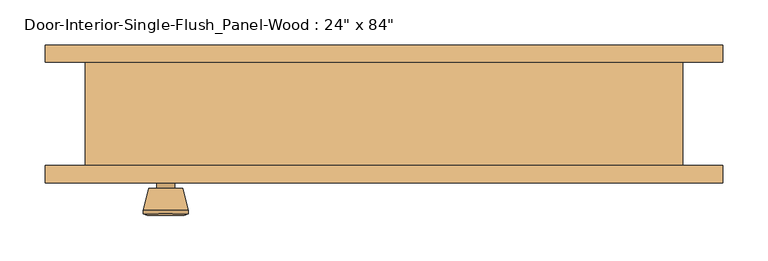
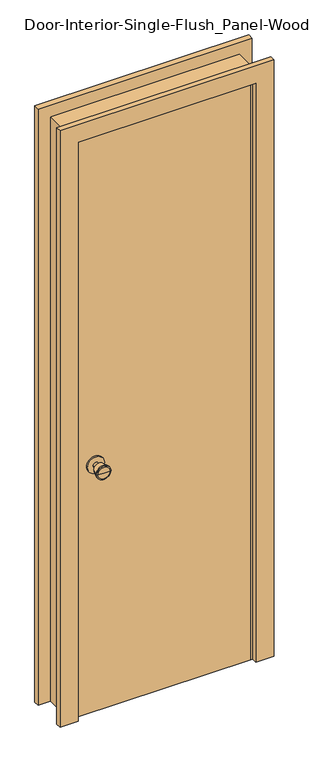
"""IFC4 building model written with IfcOpenShell, lengths in millimetres: door geometry."""

from ifc_helpers import new_model, si_unit, point, frame, frame_2d, origin, origin_with_axes, place, context, project, spatial, polyline, circle_curve, trimmed, segment, composite_curve, outline, extrude, faceted_brep, source, transform, mapped, element, save
from ifc_brep_helpers import plane_surface, cylinder_surface, revolved_surface, advanced_brep


def door_03233f92(model_context):
    return source(origin(), model_context, "Body", "SolidModel", [
        advanced_brep(
        [(-241.3, -13.05, 914.4), (-251.3, -13.05, 914.4), (-231.3, -13.05, 914.4), (-220.8241324, 35.95, 914.4), (-261.7758676, 35.95, 914.4), (-241.3, 35.95, 914.4), (-216.3, 34.1221319, 914.4), (-266.3, 34.1221319, 914.4), (-216.3, 30.6584537, 914.4), (-266.3, 30.6584537, 914.4), (-222.663764, 5.95, 914.4), (-259.936236, 5.95, 914.4), (-231.3, 5.95, 914.4), (-251.3, 5.95, 914.4)],
        [
            (0, 1),
            (1, 2, circle_curve(frame((-241.3, -13.05, 914.4), z_axis=(0.0, -1.0, 0.0), x_axis=(-1.0, 0.0, 0.0)), 10.0)),
            (2, 0),
            (2, 1, circle_curve(frame((-241.3, -13.05, 914.4), z_axis=(0.0, -1.0, 0.0), x_axis=(-1.0, 0.0, 0.0)), 10.0)),
            (3, 4, circle_curve(frame((-241.3, 35.95, 914.4), z_axis=(0.0, 1.0, 0.0), x_axis=(-1.0, 0.0, 0.0)), 20.4758676)),
            (4, 5),
            (5, 3),
            (4, 3, circle_curve(frame((-241.3, 35.95, 914.4), z_axis=(0.0, 1.0, 0.0), x_axis=(-1.0, 0.0, 0.0)), 20.4758676)),
            (6, 7, circle_curve(frame((-241.3, 34.1221319, 914.4), z_axis=(0.0, 1.0, 0.0), x_axis=(-1.0, 0.0, 0.0)), 25.0)),
            (7, 4),
            (3, 6),
            (7, 6, circle_curve(frame((-241.3, 34.1221319, 914.4), z_axis=(0.0, 1.0, 0.0), x_axis=(-1.0, 0.0, 0.0)), 25.0)),
            (8, 9, circle_curve(frame((-241.3, 30.6584537, 914.4), z_axis=(0.0, 1.0, 0.0), x_axis=(-1.0, 0.0, 0.0)), 25.0)),
            (9, 7),
            (6, 8),
            (9, 8, circle_curve(frame((-241.3, 30.6584537, 914.4), z_axis=(0.0, 1.0, 0.0), x_axis=(-1.0, 0.0, 0.0)), 25.0)),
            (10, 11, circle_curve(frame((-241.3, 5.95, 914.4), z_axis=(0.0, 1.0, 0.0), x_axis=(-1.0, 0.0, 0.0)), 18.636236)),
            (11, 9),
            (8, 10),
            (11, 10, circle_curve(frame((-241.3, 5.95, 914.4), z_axis=(0.0, 1.0, 0.0), x_axis=(-1.0, 0.0, 0.0)), 18.636236)),
            (12, 13, circle_curve(frame((-241.3, 5.95, 914.4), z_axis=(0.0, 1.0, 0.0), x_axis=(-1.0, 0.0, 0.0)), 10.0)),
            (13, 11),
            (10, 12),
            (13, 12, circle_curve(frame((-241.3, 5.95, 914.4), z_axis=(0.0, 1.0, 0.0), x_axis=(-1.0, 0.0, 0.0)), 10.0)),
            (1, 13),
            (12, 2),
        ],
        [
            plane_surface(frame((-241.3, -13.05, 914.4), z_axis=(0.0, -1.0, 0.0), x_axis=(-1.0, 0.0, 0.0))),
            plane_surface(frame((-241.3, 35.95, 914.4), z_axis=(0.0, 1.0, 0.0), x_axis=(-1.0, 0.0, 0.0))),
            revolved_surface(polyline([(-261.7758676, 35.95, 914.4), (-266.3, 34.1221319, 914.4)]), (-241.3, -13.05, 914.4), (0.0, -1.0, 0.0)),
            cylinder_surface(frame((-241.3, -13.05, 914.4), z_axis=(0.0, -1.0, 0.0), x_axis=(-1.0, 0.0, 0.0)), 25.0),
            revolved_surface(polyline([(-266.3, 30.6584537, 914.4), (-259.936236, 5.95, 914.4)]), (-241.3, -13.05, 914.4), (0.0, -1.0, 0.0)),
            plane_surface(frame((-241.3, 5.95, 914.4), z_axis=(0.0, -1.0, 0.0), x_axis=(-1.0, 0.0, 0.0))),
            cylinder_surface(frame((-241.3, -13.05, 914.4), z_axis=(0.0, -1.0, 0.0), x_axis=(-1.0, 0.0, 0.0)), 10.0),
        ],
        [
            (0, [[1, 2, 3]]),
            (0, [[-3, 4, -1]]),
            (1, [[5, 6, 7]]),
            (1, [[8, -7, -6]]),
            (2, [[9, 10, -5, 11]]),
            (2, [[12, -11, -8, -10]]),
            (3, [[13, 14, -9, 15]]),
            (3, [[16, -15, -12, -14]]),
            (4, [[17, 18, -13, 19]]),
            (4, [[20, -19, -16, -18]]),
            (5, [[21, 22, -17, 23]]),
            (5, [[24, -23, -20, -22]]),
            (6, [[-2, 25, -21, 26]]),
            (6, [[-4, -26, -24, -25]]),
        ],
    ),
        extrude(outline(composite_curve([segment(trimmed(circle_curve(frame_2d((914.4, -241.3)), 30.0), [point((914.4, -271.3))], [point((914.4, -211.3))], False, "CARTESIAN"), True, "CONTINUOUS"), segment(trimmed(circle_curve(frame_2d((914.4, -241.3)), 30.0), [point((914.4, -211.3))], [point((914.4, -271.3))], False, "CARTESIAN"), True, "CONTINUOUS")], self_intersect=False)), frame((0.0, -19.05, 0.0), z_axis=(0.0, 1.0, 0.0), x_axis=(0.0, 0.0, 1.0)), (0.0, 0.0, 1.0), 6.0),
        advanced_brep(
        [(-241.3, -59.975, 914.4), (-231.3, -59.975, 914.4), (-251.3, -59.975, 914.4), (-220.8241324, -108.975, 914.4), (-241.3, -108.975, 914.4), (-261.7758676, -108.975, 914.4), (-216.3, -107.1471319, 914.4), (-266.3, -107.1471319, 914.4), (-216.3, -103.6834537, 914.4), (-266.3, -103.6834537, 914.4), (-222.663764, -78.975, 914.4), (-259.936236, -78.975, 914.4), (-231.3, -78.975, 914.4), (-251.3, -78.975, 914.4)],
        [
            (0, 1),
            (1, 2, circle_curve(frame((-241.3, -59.975, 914.4), z_axis=(0.0, 1.0, 0.0), x_axis=(-1.0, 0.0, 0.0)), 10.0)),
            (2, 0),
            (2, 1, circle_curve(frame((-241.3, -59.975, 914.4), z_axis=(0.0, 1.0, 0.0), x_axis=(-1.0, 0.0, 0.0)), 10.0)),
            (3, 4),
            (4, 5),
            (5, 3, circle_curve(frame((-241.3, -108.975, 914.4), z_axis=(0.0, -1.0, 0.0), x_axis=(-1.0, 0.0, 0.0)), 20.4758676)),
            (3, 5, circle_curve(frame((-241.3, -108.975, 914.4), z_axis=(0.0, -1.0, 0.0), x_axis=(-1.0, 0.0, 0.0)), 20.4758676)),
            (6, 3),
            (5, 7),
            (7, 6, circle_curve(frame((-241.3, -107.1471319, 914.4), z_axis=(0.0, -1.0, 0.0), x_axis=(-1.0, 0.0, 0.0)), 25.0)),
            (6, 7, circle_curve(frame((-241.3, -107.1471319, 914.4), z_axis=(0.0, -1.0, 0.0), x_axis=(-1.0, 0.0, 0.0)), 25.0)),
            (8, 6),
            (7, 9),
            (9, 8, circle_curve(frame((-241.3, -103.6834537, 914.4), z_axis=(0.0, -1.0, 0.0), x_axis=(-1.0, 0.0, 0.0)), 25.0)),
            (8, 9, circle_curve(frame((-241.3, -103.6834537, 914.4), z_axis=(0.0, -1.0, 0.0), x_axis=(-1.0, 0.0, 0.0)), 25.0)),
            (10, 8),
            (9, 11),
            (11, 10, circle_curve(frame((-241.3, -78.975, 914.4), z_axis=(0.0, -1.0, 0.0), x_axis=(-1.0, 0.0, 0.0)), 18.636236)),
            (10, 11, circle_curve(frame((-241.3, -78.975, 914.4), z_axis=(0.0, -1.0, 0.0), x_axis=(-1.0, 0.0, 0.0)), 18.636236)),
            (12, 10),
            (11, 13),
            (13, 12, circle_curve(frame((-241.3, -78.975, 914.4), z_axis=(0.0, -1.0, 0.0), x_axis=(-1.0, 0.0, 0.0)), 10.0)),
            (12, 13, circle_curve(frame((-241.3, -78.975, 914.4), z_axis=(0.0, -1.0, 0.0), x_axis=(-1.0, 0.0, 0.0)), 10.0)),
            (1, 12),
            (13, 2),
        ],
        [
            plane_surface(frame((-241.3, -59.975, 914.4), z_axis=(0.0, 1.0, 0.0), x_axis=(-1.0, 0.0, 0.0))),
            plane_surface(frame((-241.3, -108.975, 914.4), z_axis=(0.0, -1.0, 0.0), x_axis=(-1.0, 0.0, 0.0))),
            revolved_surface(polyline([(-261.7758676, -108.975, 914.4), (-266.3, -107.1471319, 914.4)]), (-241.3, -59.975, 914.4), (0.0, 1.0, 0.0)),
            cylinder_surface(frame((-241.3, -59.975, 914.4), z_axis=(0.0, 1.0, 0.0), x_axis=(-1.0, 0.0, 0.0)), 25.0),
            revolved_surface(polyline([(-266.3, -103.6834537, 914.4), (-259.936236, -78.975, 914.4)]), (-241.3, -59.975, 914.4), (0.0, 1.0, 0.0)),
            plane_surface(frame((-241.3, -78.975, 914.4), z_axis=(0.0, 1.0, 0.0), x_axis=(-1.0, 0.0, 0.0))),
            cylinder_surface(frame((-241.3, -59.975, 914.4), z_axis=(0.0, 1.0, 0.0), x_axis=(-1.0, 0.0, 0.0)), 10.0),
        ],
        [
            (0, [[1, 2, 3]]),
            (0, [[-3, 4, -1]]),
            (1, [[5, 6, 7]]),
            (1, [[-6, -5, 8]]),
            (2, [[9, -7, 10, 11]]),
            (2, [[-10, -8, -9, 12]]),
            (3, [[13, -11, 14, 15]]),
            (3, [[-14, -12, -13, 16]]),
            (4, [[17, -15, 18, 19]]),
            (4, [[-18, -16, -17, 20]]),
            (5, [[21, -19, 22, 23]]),
            (5, [[-22, -20, -21, 24]]),
            (6, [[25, -23, 26, -2]]),
            (6, [[-26, -24, -25, -4]]),
        ],
    ),
        extrude(outline(composite_curve([segment(trimmed(circle_curve(frame_2d((914.4, -241.3)), 30.0), [point((914.4, -271.3))], [point((914.4, -211.3))], False, "CARTESIAN"), True, "CONTINUOUS"), segment(trimmed(circle_curve(frame_2d((914.4, -241.3)), 30.0), [point((914.4, -211.3))], [point((914.4, -271.3))], False, "CARTESIAN"), True, "CONTINUOUS")], self_intersect=False)), frame((0.0, -59.975, 0.0), z_axis=(0.0, 1.0, 0.0), x_axis=(0.0, 0.0, 1.0)), (0.0, 0.0, 1.0), 6.0),
        faceted_brep([(330.2, -53.975, 0.0), (304.8, -53.975, 0.0), (304.8, -19.05, 0.0), (292.1, -19.05, 0.0), (292.1, 15.875, 0.0), (304.8, 15.875, 0.0), (304.8, 60.325, 0.0), (330.2, 60.325, 0.0), (330.2, 60.325, 2159.0), (330.2, -53.975, 2159.0), (304.8, 60.325, 2133.6), (-304.8, 60.325, 2133.6), (-304.8, 60.325, 0.0), (-330.2, 60.325, 0.0), (-330.2, 60.325, 2159.0), (304.8, 15.875, 2133.6), (292.1, 15.875, 2120.9), (-292.1, 15.875, 2120.9), (-292.1, 15.875, 0.0), (-304.8, 15.875, 0.0), (-304.8, 15.875, 2133.6), (292.1, -19.05, 2120.9), (304.8, -19.05, 2133.6), (-304.8, -19.05, 2133.6), (-304.8, -19.05, 0.0), (-292.1, -19.05, 0.0), (-292.1, -19.05, 2120.9), (304.8, -53.975, 2133.6), (-330.2, -53.975, 2159.0), (-330.2, -53.975, 0.0), (-304.8, -53.975, 0.0), (-304.8, -53.975, 2133.6)], [[[0, 1, 2, 3, 4, 5, 6, 7]], [[7, 8, 9, 0]], [[6, 10, 11, 12, 13, 14, 8, 7]], [[5, 15, 10, 6]], [[4, 16, 17, 18, 19, 20, 15, 5]], [[3, 21, 16, 4]], [[2, 22, 23, 24, 25, 26, 21, 3]], [[1, 27, 22, 2]], [[0, 9, 28, 29, 30, 31, 27, 1]], [[8, 14, 28, 9]], [[15, 20, 11, 10]], [[21, 26, 17, 16]], [[27, 31, 23, 22]], [[29, 13, 12, 19, 18, 25, 24, 30]], [[14, 13, 29, 28]], [[20, 19, 12, 11]], [[26, 25, 18, 17]], [[31, 30, 24, 23]]]),
        extrude(outline(polyline([(304.8, -19.05), (304.8, -53.975), (-304.8, -53.975), (-304.8, -19.05), (304.8, -19.05)])), origin_with_axes(), (0.0, 0.0, 1.0), 2133.6),
        extrude(outline(polyline([(0.0, 374.65), (2203.45, 374.65), (2203.45, -374.65), (0.0, -374.65), (0.0, -311.15), (2139.95, -311.15), (2139.95, 311.15), (0.0, 311.15), (0.0, 374.65)])), frame((0.0, -73.025, 0.0), z_axis=(0.0, 1.0, 0.0), x_axis=(0.0, 0.0, 1.0)), (0.0, 0.0, 1.0), 19.05),
        extrude(outline(polyline([(0.0, 374.65), (2203.45, 374.65), (2203.45, -374.65), (0.0, -374.65), (0.0, -311.15), (2139.95, -311.15), (2139.95, 311.15), (0.0, 311.15), (0.0, 374.65)])), frame((0.0, 60.325, 0.0), z_axis=(0.0, 1.0, 0.0), x_axis=(0.0, 0.0, 1.0)), (0.0, 0.0, 1.0), 19.05),
    ])


if __name__ == "__main__":
    model = new_model("IFC4")
    model_context = context("Model", 3, world=origin())
    ifc_project = project(units=[si_unit("LENGTHUNIT", "METRE", prefix="MILLI")], contexts=[model_context])
    site = spatial("IfcSite", under=ifc_project)
    building = spatial("IfcBuilding", under=site)
    placement = place(None, origin())
    door_shape = door_03233f92(model_context)
    element("IfcDoor", 1, ObjectType="Door-Interior-Single-Flush_Panel-Wood : 24\" x 84\"", at=placement, inside=building, context=model_context, shape_type="MappedRepresentation", body=[
        mapped(door_shape, transform((0.0, 0.0, 0.0), x_axis=(1.0, 0.0, 0.0), y_axis=(0.0, 1.0, 0.0), z_axis=(0.0, 0.0, 1.0))),
    ])
    save(model, "model.ifc")

# Revit data of these elements
# Type "Door-Interior-Single-Flush_Panel-Wood : 24\" x 84\""
#   Type Mark = "10"
#   Assembly Code = "C1020300"
#   Analytic Construction = "Wooden"
#   Thickness = 0' - 1 3/8"
#   Thermal Resistance (R) = 2.5876 (h·ft²·°F)/BTU
#   Swing Angle [instance default] = 90.00°
#   Rough Width = 2' - 2"
#   Rough Height = 7' - 1"
#   Height = 7' - 0"
#   Width = 2' - 0"
#   Heat Transfer Coefficient (U) = 0.3865 BTU/(h·ft²·°F)
#   Trim Material = Cherry
#   Panel Material = Cherry
#   Frame Material = Cherry
#   Door Handle Material = Aluminum
#   Visual Light Transmittance = 0
#   Solar Heat Gain Coefficient = 0
#   Wall Closure = (empty or 0)
#   Function = (empty or 0)
# Element 1 (IfcDoor, "Door-Interior-Single-Flush_Panel-Wood : 24\" x 84\"")
#   Materials on its faces: "Cherry", "Aluminum"
# Materials
#   "Cherry": class "Wood", colour RGB 226 177 128, transparency 0, Description = "Prunus Serotina", Cost = 0
#   "Aluminum": class "Metal", colour RGB 247 247 247, transparency 0, Description = "Aluminum 6061", Cost = 0
